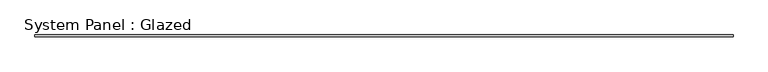
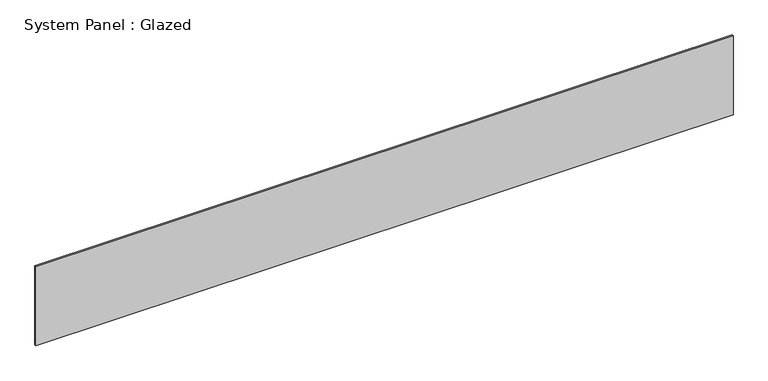
"""IFC4 building model written with IfcOpenShell, lengths in millimetres: plate geometry, System Panel : Glazed."""

from ifc_helpers import new_model, si_unit, origin, origin_with_axes, place, context, project, spatial, polyline, outline, extrude, source, transform, mapped, element, save


def system_panel_glazed_cbb493b5(model_context):
    return source(origin(), model_context, "Body", "SweptSolid", [
        extrude(outline(polyline([(5083.175, 19.05), (-5083.175, 19.05), (-5083.175, 44.45), (5083.175, 44.45), (5083.175, 19.05)])), origin_with_axes(), (0.0, 0.0, 1.0), 1219.2),
    ])


if __name__ == "__main__":
    model = new_model("IFC4")
    model_context = context("Model", 3, world=origin())
    ifc_project = project(units=[si_unit("LENGTHUNIT", "METRE", prefix="MILLI")], contexts=[model_context])
    site = spatial("IfcSite", under=ifc_project)
    building = spatial("IfcBuilding", under=site)
    placement = place(None, origin())
    system_panel_glazed_shape = system_panel_glazed_cbb493b5(model_context)
    element("IfcPlate", 1, ObjectType="System Panel : Glazed", at=placement, inside=building, context=model_context, shape_type="MappedRepresentation", body=[
        mapped(system_panel_glazed_shape, transform((0.0, 0.0, 0.0), x_axis=(1.0, 0.0, 0.0), y_axis=(0.0, 1.0, 0.0), z_axis=(0.0, 0.0, 1.0))),
    ])
    save(model, "model.ifc")

# Revit data of these elements
# Type "System Panel : Glazed"
#   Construction Type Id = "GSP4R"
#   Analytic Construction = "1/8 in Pilkington single glazing"
#   Visual Light Transmittance = 0.9
#   Solar Heat Gain Coefficient = 0.86
#   Heat Transfer Coefficient (U) = 1.18115 BTU/(h·ft²·°F)
# Element 1 (IfcPlate, "System Panel : Glazed")
#   Materials on its faces: "Glass"
# Materials
#   "Glass": class "Glass", colour RGB 0 128 192, transparency 0.75, Description = "Soda Lime Glass", Cost = 0
